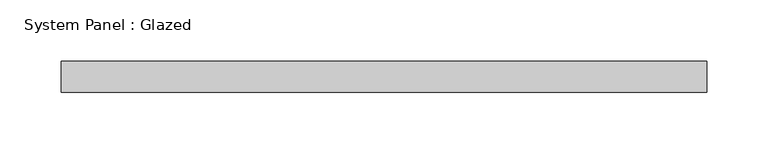
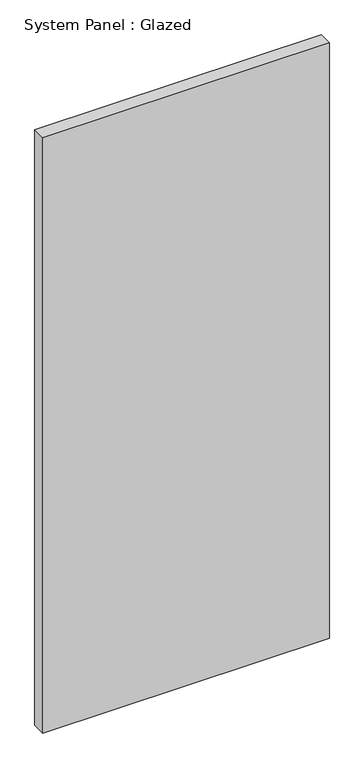
"""IFC4 building model written with IfcOpenShell, lengths in millimetres: plate geometry, System Panel : Glazed."""

from ifc_helpers import new_model, si_unit, origin, origin_with_axes, place, context, project, spatial, polyline, outline, extrude, source, transform, mapped, element, save


def system_panel_glazed_70ce58d2(model_context):
    return source(origin(), model_context, "Body", "SweptSolid", [
        extrude(outline(polyline([(263.2009491, 19.05), (-263.2009491, 19.05), (-263.2009491, 44.45), (263.2009491, 44.45), (263.2009491, 19.05)])), origin_with_axes(), (0.0, 0.0, 1.0), 1155.7),
    ])


if __name__ == "__main__":
    model = new_model("IFC4")
    model_context = context("Model", 3, world=origin())
    ifc_project = project(units=[si_unit("LENGTHUNIT", "METRE", prefix="MILLI")], contexts=[model_context])
    site = spatial("IfcSite", under=ifc_project)
    building = spatial("IfcBuilding", under=site)
    placement = place(None, origin())
    system_panel_glazed_shape = system_panel_glazed_70ce58d2(model_context)
    element("IfcPlate", 1, ObjectType="System Panel : Glazed", at=placement, inside=building, context=model_context, shape_type="MappedRepresentation", body=[
        mapped(system_panel_glazed_shape, transform((0.0, 0.0, 0.0), x_axis=(1.0, 0.0, 0.0), y_axis=(0.0, 1.0, 0.0), z_axis=(0.0, 0.0, 1.0))),
    ])
    save(model, "model.ifc")

# Revit data of these elements
# Type "System Panel : Glazed"
#   Construction Type Id = "GSP4R"
#   Analytic Construction = "1/8 in Pilkington single glazing"
#   Visual Light Transmittance = 0.9
#   Solar Heat Gain Coefficient = 0.86
#   Heat Transfer Coefficient (U) = 1.18115 BTU/(h·ft²·°F)
# Element 1 (IfcPlate, "System Panel : Glazed")
#   Materials on its faces: "Glass"
# Materials
#   "Glass": class "Glass", colour RGB 0 128 192, transparency 0.75, Description = "Soda Lime Glass", Cost = 0
